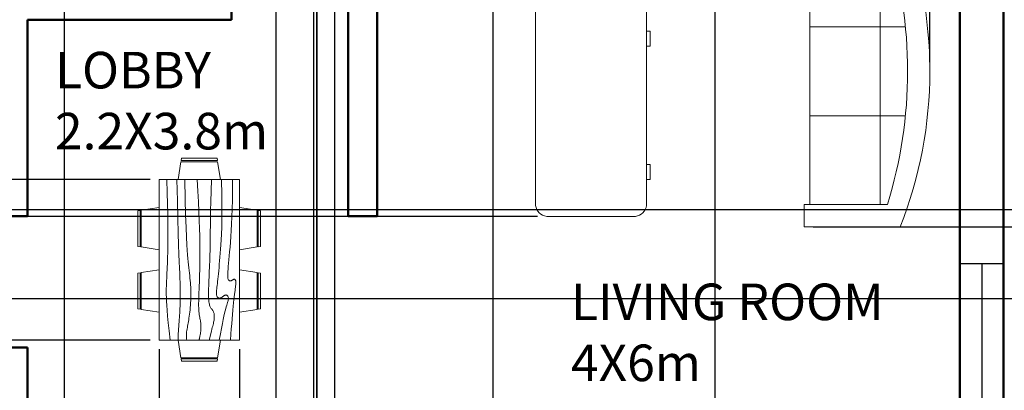
# Model space of a CAD drawing. Units: metres. Extents: x 2443.7 to 2482.9, y 2261.4 to 2287.
# Tile 4 of 8: x 2451.1 to 2457.9, y 2269.7 to 2272.3. Entities that reach past the tile are written whole.
import ezdxf

# ---------------------------------------------------------------- set-up
doc = ezdxf.new("R2010")
doc.units = ezdxf.units.M
for name, color, linetype, lineweight in [('A-ANNO-DIMS', 2, 'Continuous', 18), ('A-AREA-IDEN', 11, 'Continuous', 25), ('A-MODL', 7, 'Continuous', 25), ('A-WALL', 7, 'Continuous', 50), ('door', 6, 'Continuous', 25), ('furnitures', 20, 'Continuous', 18), ('section', 1, 'Continuous', 35), ('window', 3, 'Continuous', 25)]:
    doc.layers.add(name, color=color, linetype=linetype, lineweight=lineweight)
doc.styles.get("Standard").update_dxf_attribs({"font": 'arial.ttf'})
doc.dimstyles.get("Standard").update_dxf_attribs({"dimtxt": 0.18, "dimasz": 0.18, "dimexe": 0.18, "dimexo": 0.0625, "dimgap": 0.09, "dimtad": 0, "dimtih": 1, "dimtoh": 1, "dimdec": 4, "dimzin": 0, "dimdsep": 46, "dimtxsty": 'Standard', "dimcen": 0.09, "dimadec": 0, "dimazin": 0, "dimtfac": 1, "dimtdec": 4, "dimtofl": 0, "dimtmove": 0, "dimatfit": 3, "dimfxl": 1, "dimtolj": 1, "dimtzin": 0, "dimarcsym": 0})

# ---------------------------------------------------------------- blocks, each defined once
blk = doc.blocks.new('*U21')
for p, q in [((0, 0), (0, -6)), ((40, 0), (40, -6))]:
    blk.add_line(p, q)
blk.add_lwpolyline([(0, 0), (0, 40), (1.75, 40), (1.75, 0)], close=True)
blk.add_arc((0, 0), 40, 0, 90)
blk = doc.blocks.new('Dining Set - 36 x 72 in.')
for p, q in [((-22, 27.5), (-22.1562, 26.50042)), ((-22, 27.5), (-6, 27.5)), ((-5.8437, 26.49966), (-6, 27.5)), ((6, 27.5), (5.8438, 26.50042)), ((6, 27.5), (22, 27.5)), ((22.1563, 26.49966), (22, 27.5)), ((-22.2343, 26.00059), (-23.4847, 17.99762)), ((-22.2304, 26), (-5.7608, 26)), ((-5.8416, 26.5), (-22.1534, 26.5)), ((-4.5152, 17.99762), (-5.7655, 25.99926)), ((5.7657, 26.00059), (4.5153, 17.99762)), ((5.7696, 26), (22.2392, 26)), ((22.1584, 26.5), (5.8466, 26.5)), ((23.4848, 17.99762), (22.2345, 25.99926)), ((36, 18), (-36, 18)), ((-36, 18), (-36, -18)), ((36, -18), (36, 18)), ((-44.0006, 8.23428), (-35.9976, 9.48474)), ((44.0006, 8.23428), (35.9976, 9.48474)), ((-45.5, 8), (-44.5004, 8.15617)), ((-45.5, 8), (-45.5, -8)), ((-44.5, -8.15843), (-44.5, 8.15338)), ((-44, 8.23041), (-44, -8.23915)), ((44, 8.23041), (44, -8.23915)), ((44.5, -8.15843), (44.5, 8.15338)), ((45.5, 8), (44.5005, 8.15617)), ((45.5, 8), (45.5, -8)), ((-44.4997, -8.15631), (-45.5, -8)), ((-35.9976, -9.48476), (-43.9993, -8.2345)), ((35.9976, -9.48476), (43.9993, -8.2345)), ((44.4997, -8.15631), (45.5, -8)), ((-36, -18), (36, -18)), ((-22.2343, -26.0006), (-23.4847, -17.99762)), ((-4.5152, -17.99762), (-5.7655, -25.99928)), ((5.7657, -26.0006), (4.5153, -17.99762)), ((23.4848, -17.99762), (22.2345, -25.99928)), ((-22.2304, -26), (-5.7608, -26)), ((-22, -27.5), (-22.1562, -26.50044)), ((-5.8416, -26.5), (-22.1534, -26.5)), ((-5.8437, -26.49967), (-6, -27.5)), ((5.7696, -26), (22.2392, -26)), ((6, -27.5), (5.8438, -26.50044)), ((22.1584, -26.5), (5.8466, -26.5)), ((22.1563, -26.49967), (22, -27.5)), ((-22, -27.5), (-6, -27.5)), ((6, -27.5), (22, -27.5))]:
    blk.add_line(p, q)
for points in [[(-36, 15), (-31.1772, 14.97754), (-26.8079, 14.91406), (-22.8538, 14.81543), (-19.276, 14.6875), (-16.0362, 14.53613), (-13.0957, 14.36718), (-10.4159, 14.18652), (-7.9583, 14), (-5.6904, 13.81315), (-3.6035, 13.63021), (-1.6954, 13.45508), (0.0365, 13.29166), (1.5945, 13.14388), (2.9811, 13.01562), (4.1988, 12.9108), (5.25, 12.83333), (6.1393, 12.78613), (6.8802, 12.76823), (7.4883, 12.77767), (7.9792, 12.8125), (8.3685, 12.87077), (8.6719, 12.95052), (8.9049, 13.0498), (9.0833, 13.16666), (9.2205, 13.29899), (9.3216, 13.44401), (9.3895, 13.59879), (9.4271, 13.76041), (9.4373, 13.92594), (9.4232, 14.09245), (9.3875, 14.257), (9.3333, 14.41666), (9.2638, 14.56917), (9.1836, 14.71484), (9.0975, 14.85465), (9.0104, 14.98958), (8.9272, 15.1206), (8.8529, 15.2487), (8.7922, 15.37483), (8.75, 15.5), (8.7305, 15.62467), (8.7344, 15.74739), (8.7617, 15.86621), (8.8125, 15.97916), (8.8867, 16.08431), (8.9844, 16.17968), (9.1055, 16.26334), (9.25, 16.33333), (9.4189, 16.38802), (9.6172, 16.42708), (9.8506, 16.45052), (10.125, 16.45833), (10.4463, 16.45052), (10.8203, 16.42708), (11.2529, 16.38802), (11.75, 16.33333), (12.3184, 16.26318), (12.9694, 16.17838), (13.7151, 16.07991), (14.5677, 15.96875), (15.5395, 15.84586), (16.6426, 15.71224), (17.8893, 15.56884), (19.2917, 15.41666), (20.859, 15.25667), (22.5879, 15.08984), (24.4721, 14.91715), (26.5052, 14.73958), (28.6809, 14.5581), (30.9929, 14.3737), (33.4347, 14.18733), (36, 14)], [(-36, 10), (-28.9766, 10.14274), (-23.1725, 10.20442), (-18.4241, 10.19775), (-14.5677, 10.13541), (-11.4399, 10.03011), (-8.877, 9.89453), (-6.7154, 9.74137), (-4.7917, 9.58333), (-2.9698, 9.43082), (-1.2246, 9.28515), (0.4415, 9.14534), (2.026, 9.01041), (3.5266, 8.87939), (4.9408, 8.7513), (6.266, 8.62516), (7.5, 8.5), (8.6411, 8.37549), (9.6914, 8.2539), (10.6538, 8.13818), (11.5312, 8.03125), (12.3267, 7.93603), (13.043, 7.85547), (13.6831, 7.79248), (14.25, 7.75), (14.7471, 7.7303), (15.1797, 7.73307), (15.5537, 7.75732), (15.875, 7.80208), (16.1494, 7.86637), (16.3828, 7.94922), (16.5811, 8.04964), (16.75, 8.16666), (16.8944, 8.29915), (17.0143, 8.44531), (17.1089, 8.60319), (17.1771, 8.77083), (17.218, 8.94629), (17.2305, 9.1276), (17.2137, 9.31282), (17.1667, 9.5), (17.0895, 9.6875), (16.987, 9.875), (16.8649, 10.0625), (16.7292, 10.25), (16.5856, 10.4375), (16.4401, 10.625), (16.2985, 10.8125), (16.1667, 11), (16.05, 11.18733), (15.9518, 11.3737), (15.8752, 11.5581), (15.8229, 11.73958), (15.798, 11.91715), (15.8034, 12.08984), (15.842, 12.25667), (15.9167, 12.41666), (16.0295, 12.56836), (16.1784, 12.70833), (16.3605, 12.83268), (16.5729, 12.9375), (16.8127, 13.01888), (17.0768, 13.07291), (17.3625, 13.0957), (17.6667, 13.08333), (17.9894, 13.03312), (18.3418, 12.94726), (18.7382, 12.82918), (19.1927, 12.68229), (19.7195, 12.51001), (20.3327, 12.31575), (21.0465, 12.10294), (21.875, 11.875), (22.8357, 11.63354), (23.959, 11.37304), (25.2786, 11.08618), (26.8282, 10.76562), (28.6414, 10.40405), (30.752, 9.99414), (33.1936, 9.52856), (36, 9)], [(-36, 5.5), (-30.7157, 5.3348), (-26.069, 5.20963), (-21.9946, 5.11767), (-18.4271, 5.05208), (-15.3009, 5.00602), (-12.5508, 4.97265), (-10.1112, 4.94515), (-7.9167, 4.91666), (-5.909, 4.88167), (-4.0586, 4.83984), (-2.3429, 4.79215), (-0.7396, 4.73958), (0.7739, 4.6831), (2.22, 4.6237), (3.6213, 4.56233), (5, 4.5), (6.373, 4.43782), (7.7344, 4.3776), (9.0723, 4.32129), (10.375, 4.27083), (11.6309, 4.22819), (12.8281, 4.19531), (13.9551, 4.17415), (15, 4.16666), (15.954, 4.17448), (16.819, 4.19791), (17.6001, 4.23698), (18.3021, 4.29166), (18.9299, 4.36198), (19.4883, 4.44791), (19.9823, 4.54948), (20.4167, 4.66666), (20.7969, 4.79899), (21.1302, 4.94401), (21.4245, 5.09879), (21.6875, 5.26041), (21.9271, 5.42594), (22.1511, 5.59245), (22.3672, 5.757), (22.5834, 5.91666), (22.8065, 6.06868), (23.0404, 6.21093), (23.2879, 6.34147), (23.5521, 6.45833), (23.8358, 6.55957), (24.142, 6.64323), (24.4735, 6.70735), (24.8334, 6.75), (25.2235, 6.76969), (25.642, 6.76692), (26.0858, 6.74267), (26.5521, 6.69791), (27.0379, 6.63362), (27.5404, 6.55078), (28.0565, 6.45036), (28.5834, 6.33333), (29.1242, 6.19987), (29.7071, 6.04687), (30.3661, 5.87044), (31.1354, 5.66666), (32.0493, 5.43164), (33.142, 5.16146), (34.4475, 4.85221), (36, 4.5)], [(-36, -1), (-30.7915, -0.6591), (-26.0195, -0.38216), (-21.6519, -0.16284), (-17.6563, 0.00521), (-14.0005, 0.12833), (-10.6523, 0.21289), (-7.5796, 0.26522), (-4.75, 0.29166), (-2.134, 0.29793), (0.2878, 0.28711), (2.5317, 0.26163), (4.6146, 0.22396), (6.5529, 0.17651), (8.3633, 0.12174), (10.0623, 0.06209), (11.6667, 0), (13.1899, -0.06201), (14.6341, -0.1211), (15.9982, -0.17432), (17.2813, -0.21875), (18.4823, -0.25147), (19.6003, -0.26953), (20.6343, -0.27002), (21.5834, -0.25), (22.4481, -0.20768), (23.2357, -0.14584), (23.9549, -0.06836), (24.6146, 0.02083), (25.2235, 0.11784), (25.7904, 0.21875), (26.3241, 0.31966), (26.8334, 0.41666), (27.3265, 0.50618), (27.8099, 0.58593), (28.2894, 0.65397), (28.7709, 0.70833), (29.2601, 0.74707), (29.763, 0.76823), (30.2855, 0.76985), (30.8334, 0.75), (31.4088, 0.70784), (31.9994, 0.64713), (32.589, 0.57275), (33.1615, 0.48958), (33.7008, 0.4025), (34.1908, 0.3164), (34.6153, 0.23616), (34.9584, 0.16666), (35.2099, 0.11165), (35.3848, 0.07031), (35.504, 0.04069), (35.5886, 0.02083), (35.6594, 0.00879), (35.7377, 0.0026), (35.8442, 0.00032), (36, 0)], [(-36, -6.5), (-27.1843, -6.31267), (-20.084, -6.1263), (-14.469, -5.9419), (-10.1094, -5.76042), (-6.7752, -5.58285), (-4.2363, -5.41016), (-2.2629, -5.24333), (-0.625, -5.08334), (0.8708, -4.93099), (2.2715, -4.78646), (3.5872, -4.64974), (4.8281, -4.52084), (6.0046, -4.39974), (7.127, -4.28646), (8.2053, -4.18099), (9.25, -4.08334), (10.2705, -3.99382), (11.2734, -3.91407), (12.2647, -3.84603), (13.25, -3.79167), (14.2354, -3.75293), (15.2266, -3.73177), (16.2295, -3.73015), (17.25, -3.75), (18.2912, -3.79248), (19.3451, -3.85547), (20.4009, -3.93604), (21.4479, -4.03125), (22.4754, -4.13819), (23.4727, -4.25391), (24.4289, -4.37549), (25.3334, -4.5), (26.1785, -4.62492), (26.9694, -4.74935), (27.7145, -4.87281), (28.4219, -4.99479), (29.1, -5.11483), (29.7572, -5.23242), (30.4016, -5.34709), (31.0417, -5.45834), (31.6837, -5.56437), (32.3262, -5.65821), (32.9658, -5.73153), (33.599, -5.77604), (34.2224, -5.78345), (34.8327, -5.74545), (35.4264, -5.65373), (36, -5.5)], [(-36, -10), (-26.4022, -9.81299), (-18.4675, -9.62891), (-11.9839, -9.45069), (-6.7396, -9.28125), (-2.5226, -9.12354), (0.8789, -8.98047), (3.6769, -8.85498), (6.0833, -8.75), (8.2767, -8.66765), (10.3021, -8.60677), (12.1712, -8.56543), (13.8958, -8.54167), (15.4876, -8.53353), (16.9583, -8.53907), (18.3197, -8.55632), (19.5834, -8.58334), (20.7616, -8.61841), (21.8685, -8.66081), (22.9188, -8.71004), (23.9271, -8.76563), (24.9081, -8.82707), (25.8763, -8.89388), (26.8465, -8.96558), (27.8334, -9.04167), (28.8474, -9.12118), (29.8828, -9.20117), (30.93, -9.27824), (31.9792, -9.34896), (33.0205, -9.40991), (34.0443, -9.45768), (35.0407, -9.48885), (36, -9.5)], [(-36, -14.5), (-30.0881, -14.33513), (-25.0332, -14.21224), (-20.7312, -14.12647), (-17.0781, -14.07292), (-13.97, -14.04671), (-11.3027, -14.04297), (-8.9724, -14.05681), (-6.875, -14.08334), (-4.9224, -14.11833), (-3.0905, -14.16016), (-1.3709, -14.20785), (0.2448, -14.26042), (1.7647, -14.3169), (3.1973, -14.3763), (4.5507, -14.43767), (5.8333, -14.5), (7.0554, -14.5621), (8.235, -14.62175), (9.3922, -14.67652), (10.5469, -14.72396), (11.7192, -14.76164), (12.929, -14.78711), (14.1965, -14.79794), (15.5417, -14.79167), (16.9933, -14.76424), (18.6152, -14.70508), (20.4804, -14.60197), (22.6615, -14.44271), (25.2312, -14.21509), (28.2624, -13.9069), (31.8277, -13.50594), (36, -13)]]:
    blk.add_lwpolyline(points)
blk = doc.blocks.new('Sofa - Roundback 7 ft.')
for p, q in [((-12.00002, -32.4421), (-12.00003, -6.5971)), ((11.99997, -32.4421), (11.99998, -6.5971)), ((-36.000027, -34), (-36.000027, -11.4696)), ((35.99998, -34), (35.99998, -11.4696)), ((-35.999844, -13.3819), (35.9998, -13.3819)), ((-36.000027, -32.4421), (35.99998, -32.4421))]:
    blk.add_line(p, q)
for points in [[(-36.000027, -34), (-42.000027, -34), (-42.000027, -8)], [(41.99998, -8), (41.99998, -34), (35.99998, -34)]]:
    blk.add_lwpolyline(points)
for centre, radius, start, end in [((0, -114.25), 114.25, 68.43141, 111.5686), ((-0.00001, -127.1968), 121.1968, 72.72033, 107.2797)]:
    blk.add_arc(centre, radius, start, end)
blk = doc.blocks.new('Desk - 30 x 60 in.')
for p, q in [((-26.999995, 0), (26.999995, 0)), ((-29.999995, -27), (-29.999995, -3)), ((29.999995, -3), (29.999995, -27)), ((26.999995, -30), (-26.999995, -30)), ((-20.000005, -30), (-20.000005, -31)), ((-20.000005, -31), (-16.000005, -31)), ((-16.000005, -31), (-16.000005, -30)), ((15.999995, -31), (15.999995, -30)), ((19.999995, -31), (15.999995, -31)), ((19.999995, -30), (19.999995, -31))]:
    blk.add_line(p, q)
for centre, start, end in [((-26.499995, -3.5), 98.1301, 171.8699), ((26.499995, -3.5), 8.130102, 81.8699), ((-26.499995, -26.5), 188.1301, 261.8699), ((26.499995, -26.5), 278.1301, 351.8699)]:
    blk.add_arc(centre, 3.535534, start, end)
blk = doc.blocks.new('aditya')
at = {"layer": 'A-WALL'}
for p, q in [((10.2, 3.3), (10.2, 9.9)), ((5.9, 6.0521), (5.9, 9.6)), ((9.9, 5), (9.9, 9.6)), ((5.7, 6.0521), (5.7, 8.5)), ((4.9, 7.4), (4.9, 7.6734)), ((3.5, 6.0521), (3.5, 7.4)), ((3.5, 7.4), (4.9, 7.4)), ((5.7, 6.0521), (5.9, 6.0521)), ((3.5, 4.4718), (3.5, 5.1521)), ((9.9, 4.8), (9.9, 5))]:
    blk.add_line(p, q, dxfattribs=at)
for points in [[(3.3, 6.0498), (3.3, 6.0521), (3.5, 6.0521)], [(3.5, 5.1521), (3.3, 5.1521), (3.3, 5.1915)]]:
    blk.add_lwpolyline(points, dxfattribs=at)
at = {"layer": 'section'}
blk.add_line((5.4866, -1.5581), (5.4866, 11.3875), dxfattribs=at)
at = {"layer": 'window'}
blk.add_line((10.05, 5.7272), (10.05, 4.5272), dxfattribs=at)
blk.add_lwpolyline([(9.9, 5.7272), (10.2, 5.7272), (10.2, 4.5272), (9.9, 4.5272)], close=True, dxfattribs=at)
at = {"layer": 'door', "xscale": 0.0224999999999983, "yscale": 0.0224999999999983, "zscale": 0.0224999999999983, "rotation": 90}
blk.add_blockref('*U21', (3.365, 5.1521), dxfattribs=at)
at = {"layer": 'furnitures'}
for name, p, xscale, yscale, zscale, rotation in [('Sofa - Roundback 7 ft.', (9.6938, 7.0466), 0.0254, 0.0254, 0.0254, 270), ('Desk - 30 x 60 in.', (6.9873, 6.8124), 0.0254, 0.0254, 0.0254, 90), ('Dining Set - 36 x 72 in.', (4.6784, 5.7534), 0.0152922016691108, 0.0152922016691108, 0.0152922016691108, 270)]:
    blk.add_blockref(name, p, dxfattribs=dict(at, xscale=xscale, yscale=yscale, zscale=zscale, rotation=rotation))
at = {"layer": 'A-AREA-IDEN', "char_height": 0.250924, "attachment_point": 1}
for s, insert in [('{\\fArial|b1|i1|c0|p34;LOBBY\\P2.2X3.8m}', (3.6877, 7.1796)), ('{\\fArial|b1|i1|c0|p34;LIVING ROOM\\P4X6m}', (7.2298, 5.5901))]:
    blk.add_mtext_dynamic_manual_height_columns(s, width=10.569305, gutter_width=7.8414, heights=[0], dxfattribs=dict(at, insert=insert))
blk = doc.blocks.new('*D23')
at = {"layer": 'A-ANNO-DIMS', "color": 0, "lineweight": -2, "transparency": 16777216}
for p, q in [((2457.9453, 2274.7597), (2482.2428, 2274.7597)), ((2482.0628, 2274.5797), (2482.0628, 2269.6416)), ((2482.0628, 2264.3397), (2482.0628, 2269.2778)), ((2453.6453, 2264.1597), (2482.2428, 2264.1597))]:
    blk.add_line(p, q, dxfattribs=at)
at = {"layer": 'A-ANNO-DIMS', "color": 0, "transparency": 16777216}
for points in [[(2482.0328, 2274.5797), (2482.0928, 2274.5797), (2482.0628, 2274.7597)], [(2482.0328, 2264.3397), (2482.0928, 2264.3397), (2482.0628, 2264.1597)]]:
    blk.add_solid(points, dxfattribs=at)
at = {"layer": 'Defpoints', "color": 0, "transparency": 16777216}
for p in [(2457.8828, 2274.7597), (2453.5828, 2264.1597), (2482.0628, 2264.1597)]:
    blk.add_point(p, dxfattribs=at)
at = {"layer": 'A-ANNO-DIMS', "color": 0, "transparency": 16777216, "insert": (2482.0628, 2269.4597), "char_height": 0.18, "attachment_point": 5}
blk.add_mtext('\\A1;10.6', dxfattribs=at)
blk = doc.blocks.new('*D35')
at = {"layer": 'A-ANNO-DIMS', "color": 0, "lineweight": -2, "transparency": 16777216}
for p, q in [((2457.9453, 2272.3017), (2482.2428, 2272.3017)), ((2482.0628, 2272.1217), (2482.0628, 2271.6247)), ((2482.0628, 2270.7669), (2482.0628, 2271.2639)), ((2457.9453, 2270.5869), (2482.2428, 2270.5869))]:
    blk.add_line(p, q, dxfattribs=at)
at = {"layer": 'A-ANNO-DIMS', "color": 0, "transparency": 16777216}
for points in [[(2482.0328, 2272.1217), (2482.0928, 2272.1217), (2482.0628, 2272.3017)], [(2482.0328, 2270.7669), (2482.0928, 2270.7669), (2482.0628, 2270.5869)]]:
    blk.add_solid(points, dxfattribs=at)
at = {"layer": 'Defpoints', "color": 0, "transparency": 16777216}
for p in [(2457.8828, 2272.3017), (2457.8828, 2270.5869), (2482.0628, 2270.5869)]:
    blk.add_point(p, dxfattribs=at)
at = {"layer": 'A-ANNO-DIMS', "color": 0, "transparency": 16777216, "insert": (2482.0628, 2271.4443), "char_height": 0.18, "attachment_point": 5}
blk.add_mtext('\\A1;1.71', dxfattribs=at)
blk = doc.blocks.new('*D38')
at = {"layer": 'A-ANNO-DIMS', "color": 0, "lineweight": -2, "transparency": 16777216}
for p, q in [((2454.3757, 2273.1253), (2454.3757, 2261.3876)), ((2455.8997, 2273.1253), (2455.8997, 2261.3876)), ((2454.5557, 2261.5676), (2454.7528, 2261.5676)), ((2455.7197, 2261.5676), (2455.5225, 2261.5676))]:
    blk.add_line(p, q, dxfattribs=at)
at = {"layer": 'A-ANNO-DIMS', "color": 0, "transparency": 16777216}
for points in [[(2454.5557, 2261.5976), (2454.5557, 2261.5376), (2454.3757, 2261.5676)], [(2455.7197, 2261.5976), (2455.7197, 2261.5376), (2455.8997, 2261.5676)]]:
    blk.add_solid(points, dxfattribs=at)
at = {"layer": 'Defpoints', "color": 0, "transparency": 16777216}
for p in [(2454.3757, 2273.1878), (2455.8997, 2273.1878), (2454.3757, 2261.5676)]:
    blk.add_point(p, dxfattribs=at)
at = {"layer": 'A-ANNO-DIMS', "color": 0, "transparency": 16777216, "insert": (2455.1377, 2261.5676), "char_height": 0.18, "attachment_point": 5}
blk.add_mtext('\\A1;1.524', dxfattribs=at)
blk = doc.blocks.new('*D40')
at = {"layer": 'A-ANNO-DIMS', "color": 0, "lineweight": -2, "transparency": 16777216}
for p, q in [((2456.5754, 2272.973), (2482.2428, 2272.973)), ((2482.0628, 2272.793), (2482.0628, 2272.0882)), ((2482.0628, 2271.0194), (2482.0628, 2271.7243)), ((2456.5754, 2270.8394), (2482.2428, 2270.8394))]:
    blk.add_line(p, q, dxfattribs=at)
at = {"layer": 'A-ANNO-DIMS', "color": 0, "transparency": 16777216}
for points in [[(2482.0328, 2272.793), (2482.0928, 2272.793), (2482.0628, 2272.973)], [(2482.0328, 2271.0194), (2482.0928, 2271.0194), (2482.0628, 2270.8394)]]:
    blk.add_solid(points, dxfattribs=at)
at = {"layer": 'Defpoints', "color": 0, "transparency": 16777216}
for p in [(2456.5129, 2272.973), (2482.0628, 2272.973), (2456.5129, 2270.8394)]:
    blk.add_point(p, dxfattribs=at)
at = {"layer": 'A-ANNO-DIMS', "color": 0, "transparency": 16777216, "insert": (2482.0628, 2271.9062), "char_height": 0.18, "attachment_point": 5}
blk.add_mtext('\\A1;2.13', dxfattribs=at)
blk = doc.blocks.new('*D41')
at = {"layer": 'A-ANNO-DIMS', "color": 0, "lineweight": -2, "transparency": 16777216}
for p, q in [((2456.512931, 2273.035548), (2456.512931, 2287.015188)), ((2457.376531, 2271.968748), (2457.376531, 2287.015188)), ((2456.332931, 2286.835188), (2456.152931, 2286.835188)), ((2457.556531, 2286.835188), (2457.736531, 2286.835188))]:
    blk.add_line(p, q, dxfattribs=at)
at = {"layer": 'A-ANNO-DIMS', "color": 0, "transparency": 16777216}
for points in [[(2456.332931, 2286.865188), (2456.332931, 2286.805188), (2456.512931, 2286.835188)], [(2457.556531, 2286.865188), (2457.556531, 2286.805188), (2457.376531, 2286.835188)]]:
    blk.add_solid(points, dxfattribs=at)
at = {"layer": 'Defpoints', "color": 0, "transparency": 16777216}
for p in [(2457.376531, 2286.835188), (2456.512931, 2272.973048), (2457.376531, 2271.906248)]:
    blk.add_point(p, dxfattribs=at)
at = {"layer": 'A-ANNO-DIMS', "color": 0, "transparency": 16777216, "insert": (2456.944731, 2286.835188), "char_height": 0.18, "attachment_point": 5}
blk.add_mtext('\\A1;0.86', dxfattribs=at)
blk = doc.blocks.new('*D42')
at = {"layer": 'A-ANNO-DIMS', "color": 0, "lineweight": -2, "transparency": 16777216}
for p, q in [((2454.6838, 2272.434), (2444.1027, 2272.434)), ((2444.2827, 2272.254), (2444.2827, 2271.854)), ((2444.2827, 2271.09), (2444.2827, 2271.4901)), ((2454.6838, 2270.91), (2444.1027, 2270.91))]:
    blk.add_line(p, q, dxfattribs=at)
at = {"layer": 'A-ANNO-DIMS', "color": 0, "transparency": 16777216}
for points in [[(2444.2527, 2272.254), (2444.3127, 2272.254), (2444.2827, 2272.434)], [(2444.2527, 2271.09), (2444.3127, 2271.09), (2444.2827, 2270.91)]]:
    blk.add_solid(points, dxfattribs=at)
at = {"layer": 'Defpoints', "color": 0, "transparency": 16777216}
for p in [(2444.2827, 2272.434), (2454.7463, 2272.434), (2454.7463, 2270.91)]:
    blk.add_point(p, dxfattribs=at)
at = {"layer": 'A-ANNO-DIMS', "color": 0, "transparency": 16777216, "insert": (2444.2827, 2271.672), "char_height": 0.18, "attachment_point": 5}
blk.add_mtext('\\A1;1.524', dxfattribs=at)
blk = doc.blocks.new('*D44')
at = {"layer": 'A-ANNO-DIMS', "color": 0, "lineweight": -2, "transparency": 16777216}
for p, q in [((2452.0859, 2270), (2452.0859, 2261.3876)), ((2452.6364, 2270), (2452.6364, 2261.3876)), ((2452.2659, 2261.5676), (2452.4564, 2261.5676)), ((2452.6364, 2261.5676), (2452.8164, 2261.5676))]:
    blk.add_line(p, q, dxfattribs=at)
at = {"layer": 'A-ANNO-DIMS', "color": 0, "transparency": 16777216}
for points in [[(2452.2659, 2261.5976), (2452.2659, 2261.5376), (2452.0859, 2261.5676)], [(2452.4564, 2261.5976), (2452.4564, 2261.5376), (2452.6364, 2261.5676)]]:
    blk.add_solid(points, dxfattribs=at)
at = {"layer": 'Defpoints', "color": 0, "transparency": 16777216}
for p in [(2452.0859, 2270.0625), (2452.6364, 2270.0625), (2452.6364, 2261.5676)]:
    blk.add_point(p, dxfattribs=at)
at = {"layer": 'A-ANNO-DIMS', "color": 0, "transparency": 16777216, "insert": (2453.1409, 2261.5676), "char_height": 0.18, "attachment_point": 5}
blk.add_mtext('\\A1;0.55', dxfattribs=at)
blk = doc.blocks.new('*D45')
at = {"layer": 'A-ANNO-DIMS', "color": 0, "lineweight": -2, "transparency": 16777216}
for p, q in [((2452.0234, 2271.1636), (2444.1027, 2271.1636)), ((2444.2827, 2270.9836), (2444.2827, 2270.795)), ((2444.2827, 2270.2425), (2444.2827, 2270.4312)), ((2452.0234, 2270.0625), (2444.1027, 2270.0625))]:
    blk.add_line(p, q, dxfattribs=at)
at = {"layer": 'A-ANNO-DIMS', "color": 0, "transparency": 16777216}
for points in [[(2444.2527, 2270.9836), (2444.3127, 2270.9836), (2444.2827, 2271.1636)], [(2444.2527, 2270.2425), (2444.3127, 2270.2425), (2444.2827, 2270.0625)]]:
    blk.add_solid(points, dxfattribs=at)
at = {"layer": 'Defpoints', "color": 0, "transparency": 16777216}
for p in [(2444.2827, 2271.1636), (2452.0859, 2271.1636), (2452.0859, 2270.0625)]:
    blk.add_point(p, dxfattribs=at)
at = {"layer": 'A-ANNO-DIMS', "color": 0, "transparency": 16777216, "insert": (2444.2827, 2270.6131), "char_height": 0.18, "attachment_point": 5}
blk.add_mtext('\\A1;1.101', dxfattribs=at)
blk = doc.blocks.new('*D55')
at = {"layer": 'A-ANNO-DIMS', "color": 0, "lineweight": -2, "transparency": 16777216}
for p, q in [((2452.8879, 2274.2987), (2452.8879, 2261.3876)), ((2453.1465, 2274.2987), (2453.1465, 2261.3876)), ((2452.7079, 2261.5676), (2452.5279, 2261.5676)), ((2453.3265, 2261.5676), (2453.5065, 2261.5676))]:
    blk.add_line(p, q, dxfattribs=at)
at = {"layer": 'A-ANNO-DIMS', "color": 0, "transparency": 16777216}
for points in [[(2452.7079, 2261.5976), (2452.7079, 2261.5376), (2452.8879, 2261.5676)], [(2453.3265, 2261.5976), (2453.3265, 2261.5376), (2453.1465, 2261.5676)]]:
    blk.add_solid(points, dxfattribs=at)
at = {"layer": 'Defpoints', "color": 0, "transparency": 16777216}
for p in [(2452.8879, 2274.3612), (2453.1465, 2274.3612), (2453.1465, 2261.5676)]:
    blk.add_point(p, dxfattribs=at)
at = {"layer": 'A-ANNO-DIMS', "color": 0, "transparency": 16777216, "insert": (2453.8302, 2261.5676), "char_height": 0.18, "attachment_point": 5}
blk.add_mtext('\\A1;0.26', dxfattribs=at)
blk = doc.blocks.new('*D58')
at = {"layer": 'A-ANNO-DIMS', "color": 0, "lineweight": -2, "transparency": 16777216}
for p, q in [((2448.7151, 2270.9583), (2482.2428, 2270.9583)), ((2482.0628, 2270.7783), (2482.0628, 2270.5266)), ((2448.7277, 2270.3466), (2482.2428, 2270.3466)), ((2482.0628, 2270.3466), (2482.0628, 2270.1666)), ((2482.0628, 2270.1666), (2481.8828, 2270.1666))]:
    blk.add_line(p, q, dxfattribs=at)
at = {"layer": 'A-ANNO-DIMS', "color": 0, "transparency": 16777216}
for points in [[(2482.0328, 2270.7783), (2482.0928, 2270.7783), (2482.0628, 2270.9583)], [(2482.0328, 2270.5266), (2482.0928, 2270.5266), (2482.0628, 2270.3466)]]:
    blk.add_solid(points, dxfattribs=at)
at = {"layer": 'Defpoints', "color": 0, "transparency": 16777216}
for p in [(2448.6526, 2270.9583), (2448.6652, 2270.3466), (2482.0628, 2270.3466)]:
    blk.add_point(p, dxfattribs=at)
at = {"layer": 'A-ANNO-DIMS', "color": 0, "transparency": 16777216, "insert": (2481.5764, 2270.1666), "char_height": 0.18, "attachment_point": 5}
blk.add_mtext('\\A1;0.61', dxfattribs=at)
blk = doc.blocks.new('*D63')
at = {"layer": 'A-ANNO-DIMS', "color": 0, "lineweight": -2, "transparency": 16777216}
for p, q in [((2447.6828, 2278.9987), (2447.6828, 2261.3876)), ((2457.8828, 2278.9987), (2457.8828, 2261.3876)), ((2447.8628, 2261.5676), (2452.4684, 2261.5676)), ((2457.7028, 2261.5676), (2453.0971, 2261.5676))]:
    blk.add_line(p, q, dxfattribs=at)
at = {"layer": 'A-ANNO-DIMS', "color": 0, "transparency": 16777216}
for points in [[(2447.8628, 2261.5976), (2447.8628, 2261.5376), (2447.6828, 2261.5676)], [(2457.7028, 2261.5976), (2457.7028, 2261.5376), (2457.8828, 2261.5676)]]:
    blk.add_solid(points, dxfattribs=at)
at = {"layer": 'Defpoints', "color": 0, "transparency": 16777216}
for p in [(2447.6828, 2279.0612), (2457.8828, 2279.0612), (2457.8828, 2261.5676)]:
    blk.add_point(p, dxfattribs=at)
at = {"layer": 'A-ANNO-DIMS', "color": 0, "transparency": 16777216, "insert": (2452.7828, 2261.5676), "char_height": 0.18, "attachment_point": 5}
blk.add_mtext('\\A1;10.2', dxfattribs=at)
blk = doc.blocks.new('*D71')
at = {"layer": 'A-ANNO-DIMS', "color": 0, "lineweight": -2, "transparency": 16777216}
for p, q in [((2451.4341, 2281.6186), (2451.4341, 2261.3876)), ((2453.2904, 2281.6186), (2453.2904, 2261.3876)), ((2451.6141, 2261.5676), (2452.047, 2261.5676)), ((2453.1104, 2261.5676), (2452.6775, 2261.5676))]:
    blk.add_line(p, q, dxfattribs=at)
at = {"layer": 'A-ANNO-DIMS', "color": 0, "transparency": 16777216}
for points in [[(2451.6141, 2261.5976), (2451.6141, 2261.5376), (2451.4341, 2261.5676)], [(2453.1104, 2261.5976), (2453.1104, 2261.5376), (2453.2904, 2261.5676)]]:
    blk.add_solid(points, dxfattribs=at)
at = {"layer": 'Defpoints', "color": 0, "transparency": 16777216}
for p in [(2451.4341, 2281.6811), (2453.2904, 2281.6811), (2453.2904, 2261.5676)]:
    blk.add_point(p, dxfattribs=at)
at = {"layer": 'A-ANNO-DIMS', "color": 0, "transparency": 16777216, "insert": (2452.3623, 2261.5676), "char_height": 0.18, "attachment_point": 5}
blk.add_mtext('\\A1;1.86', dxfattribs=at)

msp = doc.modelspace()

# ---------------------------------------------------------------- block references
at = {"layer": 'A-MODL'}
msp.add_blockref('aditya', (2447.682762, 2264.859673), dxfattribs=at)

# ---------------------------------------------------------------- dimensions: what is measured, and where the dimension line sits
at = {"layer": 'A-ANNO-DIMS'}
for base, p1, p2, override, picture, middle in [((2457.376531, 2286.835188), (2456.512931, 2272.973048), (2457.376531, 2271.906248), {"dimdec": 2, "dimlfac": 1, "dimrnd": 0, "dimzin": 0, "dimdsep": 46, "dimlunit": 2}, '*D41', (2456.944731, 2286.835188)), ((2453.29044, 2261.567605), (2451.43413, 2281.681077), (2453.29044, 2281.681077), {"dimdec": 2, "dimlfac": 1, "dimrnd": 0, "dimzin": 0, "dimdsep": 46, "dimlunit": 2}, '*D71', (2452.362285, 2261.567605)), ((2457.882762, 2261.567605), (2447.682762, 2279.061188), (2457.882762, 2279.061188), {"dimdec": 1, "dimlfac": 1, "dimrnd": 0, "dimzin": 0, "dimdsep": 46, "dimlunit": 2}, '*D63', (2452.782762, 2261.567605)), ((2453.146499, 2261.567605), (2452.887881, 2274.361152), (2453.146499, 2274.361152), {"dimdec": 2, "dimlfac": 1, "dimrnd": 0, "dimzin": 0, "dimdsep": 46, "dimlunit": 2}, '*D55', (2453.830217, 2261.567605)), ((2454.375659, 2261.567605), (2455.89966, 2273.187816), (2454.375659, 2273.187816), {"dimdec": 3, "dimlfac": 1, "dimrnd": 0, "dimzin": 0, "dimdsep": 46, "dimlunit": 2}, '*D38', (2455.13766, 2261.567605)), ((2452.636436, 2261.567605), (2452.085916, 2270.062544), (2452.636436, 2270.062544), {"dimdec": 2, "dimlfac": 1, "dimrnd": 0, "dimzin": 0, "dimdsep": 46, "dimlunit": 2}, '*D44', (2453.14089, 2261.567605))]:
    dim = msp.add_linear_dim(base=base, p1=p1, p2=p2, dimstyle='Standard', override=override, dxfattribs=at)
    dim.commit()
    dim.dimension.update_dxf_attribs({"geometry": picture, "text_midpoint": middle})
for base, p1, p2, override, picture, middle in [((2482.062768, 2264.159673), (2457.882762, 2274.759673), (2453.582762, 2264.159673), {"dimdec": 1, "dimlfac": 1, "dimrnd": 0, "dimzin": 0, "dimdsep": 46, "dimlunit": 2}, '*D23', (2482.062768, 2269.459673)), ((2482.062768, 2272.973048), (2456.512931, 2270.839448), (2456.512931, 2272.973048), {"dimdec": 2, "dimlfac": 1, "dimrnd": 0, "dimzin": 0, "dimdsep": 46, "dimlunit": 2}, '*D40', (2482.062768, 2271.906248)), ((2444.282724, 2272.434047), (2454.746253, 2270.910047), (2454.746253, 2272.434047), {"dimdec": 3, "dimlfac": 1, "dimrnd": 0, "dimzin": 0, "dimdsep": 46, "dimlunit": 2}, '*D42', (2444.282724, 2271.672047)), ((2482.062768, 2270.586919), (2457.882762, 2272.301681), (2457.882762, 2270.586919), {"dimdec": 2, "dimlfac": 1, "dimrnd": 0, "dimzin": 0, "dimdsep": 46, "dimlunit": 2}, '*D35', (2482.062768, 2271.4443)), ((2444.282724, 2271.163582), (2452.085916, 2270.062544), (2452.085916, 2271.163582), {"dimdec": 3, "dimlfac": 1, "dimrnd": 0, "dimzin": 0, "dimdsep": 46, "dimlunit": 2}, '*D45', (2444.282724, 2270.613063)), ((2482.062768, 2270.346637), (2448.652642, 2270.958301), (2448.665238, 2270.346637), {"dimdec": 2, "dimlfac": 1, "dimrnd": 0, "dimzin": 0, "dimdsep": 46, "dimlunit": 2}, '*D58', (2481.576363, 2270.166637))]:
    dim = msp.add_linear_dim(base=base, p1=p1, p2=p2, angle=90, dimstyle='Standard', override=override, dxfattribs=at)
    dim.commit()
    dim.dimension.update_dxf_attribs({"geometry": picture, "text_midpoint": middle})

doc.saveas('drawing.dxf')
